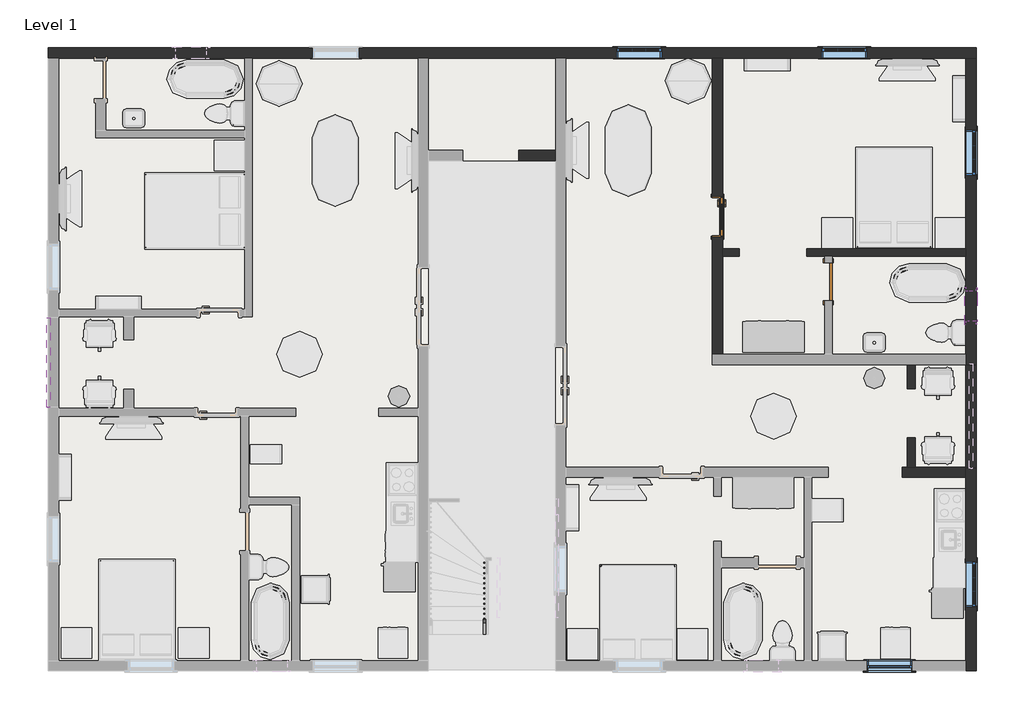
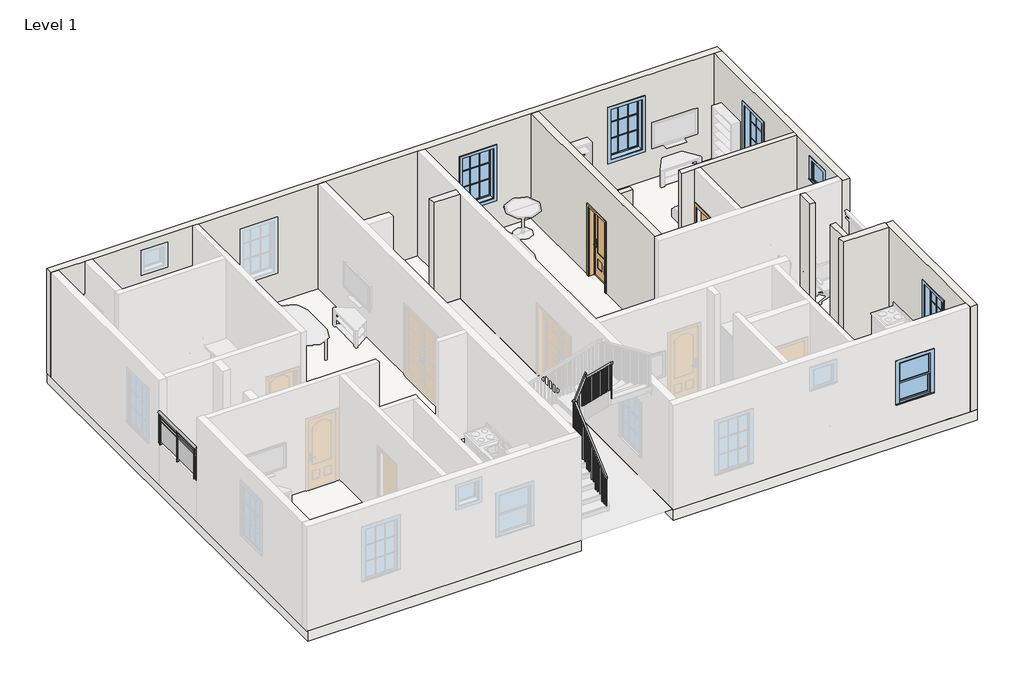
# One storey, part 2 of 4: 11 walls, 6 windows, 2 doors, 2 railings, 1 slab.
"""IFC4 building model written with IfcOpenShell, lengths in millimetres."""

from ifc_helpers import new_model, si_unit, point, frame, origin, origin_with_axes, place, context, project, spatial, polyline, ellipse_curve, trimmed, outline, extrude, faceted_brep, transform, mapped, element, save
from ifc_brep_helpers import plane_surface, extruded_surface, advanced_brep
from components import door_41326d50, door_255cab33, window_58e1470a, window_31198920, window_e41d21a6

model = new_model("IFC4")

# Units and contexts
model_context = context("Model", 3, world=origin())
ifc_project = project(units=[si_unit("LENGTHUNIT", "METRE", prefix="MILLI")], contexts=[model_context])

# Site, building, storey
site = spatial("IfcSite", under=ifc_project)
building = spatial("IfcBuilding", under=site)
storey = spatial("IfcBuildingStorey", under=building, Name="Level 1", Elevation=0.0)

# Doors
placement = place(None, origin())
door_shape = door_41326d50(model_context)
element("IfcDoor", 1, ObjectType="30\" x 80\"", at=placement, inside=storey, context=model_context, shape_type="MappedRepresentation", body=[
    mapped(door_shape, transform((-3299.0058972, 9528.0923354, 0.0), x_axis=(0.0, 1.0, 0.0), y_axis=(-1.0, 0.0, 0.0), z_axis=(0.0, 0.0, 1.0))),
])
door_2_shape = door_255cab33(model_context)
element("IfcDoor", 2, ObjectType="Single-Flush : 30\" x 80\"", at=placement, inside=storey, context=model_context, shape_type="MappedRepresentation", body=[
    mapped(door_2_shape, transform((-1092.3808972, 8232.6923354, 0.0), x_axis=(0.0, 1.0, 0.0), y_axis=(-1.0, 0.0, 0.0), z_axis=(0.0, 0.0, 1.0))),
])

# Railings
element("IfcRailing", 3, ObjectType="Glass Panel - Bottom Fill", at=placement, inside=storey, context=model_context, shape_type="SolidModel", body=[
    advanced_brep(
    [(-16599.0808972, 7508.7923354, 2133.6), (-16675.2808972, 7508.7923354, 2133.6), (-16599.0808972, 5730.7923354, 2133.6), (-16675.2808972, 5730.7923354, 2133.6)],
    [
        (0, 1, ellipse_curve(frame((-16637.1808972, 7508.7923354, 2133.6), z_axis=(0.0, 1.0, 0.0), x_axis=(-1.0, 0.0, 0.0)), 38.1, 28.575)),
        (1, 0, ellipse_curve(frame((-16637.1808972, 7508.7923354, 2133.6), z_axis=(0.0, 1.0, 0.0), x_axis=(-1.0, 0.0, 0.0)), 38.1, 28.575)),
        (2, 3, ellipse_curve(frame((-16637.1808972, 5730.7923354, 2133.6), z_axis=(0.0, -1.0, 0.0), x_axis=(-1.0, 0.0, 0.0)), 38.1, 28.575)),
        (3, 2, ellipse_curve(frame((-16637.1808972, 5730.7923354, 2133.6), z_axis=(0.0, -1.0, 0.0), x_axis=(-1.0, 0.0, 0.0)), 38.1, 28.575)),
        (0, 2),
        (3, 1),
    ],
    [
        plane_surface(frame((-16637.1808972, 7508.7923354, 2133.6), z_axis=(0.0, 1.0, 0.0), x_axis=(0.0, 0.0, -1.0))),
        plane_surface(frame((-16637.1808972, 5730.7923354, 2133.6), z_axis=(0.0, -1.0, 0.0), x_axis=(0.0, 0.0, -1.0))),
        extruded_surface(trimmed(ellipse_curve(frame((-16637.1808972, 5730.7923354, 2133.6), z_axis=(0.0, 1.0, 0.0), x_axis=(-1.0, 0.0, 0.0)), 38.1, 28.575), [point((-16599.0808972, 5730.7923354, 2133.6))], [point((-16675.2808972, 5730.7923354, 2133.6))], True, "CARTESIAN"), (0.0, 1778.0, 0.0), 1778.0),
        extruded_surface(trimmed(ellipse_curve(frame((-16637.1808972, 5730.7923354, 2133.6), z_axis=(0.0, 1.0, 0.0), x_axis=(-1.0, 0.0, 0.0)), 38.1, 28.575), [point((-16675.2808972, 5730.7923354, 2133.6))], [point((-16599.0808972, 5730.7923354, 2133.6))], True, "CARTESIAN"), (0.0, 1778.0, 0.0), 1778.0),
    ],
    [
        (0, [[1, 2]]),
        (1, [[3, 4]]),
        (2, [[-1, 5, -4, 6]]),
        (3, [[-2, -6, -3, -5]]),
    ],
),
    extrude(outline(polyline([(-16649.8808972, 7508.7923354), (-16624.4808972, 7508.7923354), (-16624.4808972, 5730.7923354), (-16649.8808972, 5730.7923354), (-16649.8808972, 7508.7923354)])), frame((0.0, 0.0, 2019.3), z_axis=(0.0, 0.0, 1.0), x_axis=(1.0, 0.0, 0.0)), (0.0, 0.0, 1.0), 25.4),
    extrude(outline(polyline([(-16649.8808972, 7508.7923354), (-16624.4808972, 7508.7923354), (-16624.4808972, 5730.7923354), (-16649.8808972, 5730.7923354), (-16649.8808972, 7508.7923354)])), frame((0.0, 0.0, 1917.7), z_axis=(0.0, 0.0, 1.0), x_axis=(1.0, 0.0, 0.0)), (0.0, 0.0, 1.0), 25.4),
    extrude(outline(polyline([(-16662.5808972, 5813.3423354), (-16611.7808972, 5813.3423354), (-16611.7808972, 5800.6423354), (-16662.5808972, 5800.6423354), (-16662.5808972, 5813.3423354)])), frame((0.0, 0.0, 1219.2), z_axis=(0.0, 0.0, 1.0), x_axis=(1.0, 0.0, 0.0)), (0.0, 0.0, 1.0), 885.6788223),
    extrude(outline(polyline([(-16630.6457402, 6619.7923354), (-16630.6457402, 5806.9923354), (-16636.9957402, 5806.9923354), (-16636.9957402, 6619.7923354), (-16630.6457402, 6619.7923354)])), frame((0.0, 0.0, 1320.8), z_axis=(0.0, 0.0, 1.0), x_axis=(1.0, 0.0, 0.0)), (0.0, 0.0, 1.0), 596.9),
    extrude(outline(polyline([(-16662.5808972, 6626.1423354), (-16611.7808972, 6626.1423354), (-16611.7808972, 6613.4423354), (-16662.5808972, 6613.4423354), (-16662.5808972, 6626.1423354)])), frame((0.0, 0.0, 1219.2), z_axis=(0.0, 0.0, 1.0), x_axis=(1.0, 0.0, 0.0)), (0.0, 0.0, 1.0), 885.6788223),
    extrude(outline(polyline([(-16630.6457402, 7432.5923354), (-16630.6457402, 6619.7923354), (-16636.9957402, 6619.7923354), (-16636.9957402, 7432.5923354), (-16630.6457402, 7432.5923354)])), frame((0.0, 0.0, 1320.8), z_axis=(0.0, 0.0, 1.0), x_axis=(1.0, 0.0, 0.0)), (0.0, 0.0, 1.0), 596.9),
    extrude(outline(polyline([(-16662.5808972, 7438.9423354), (-16611.7808972, 7438.9423354), (-16611.7808972, 7426.2423354), (-16662.5808972, 7426.2423354), (-16662.5808972, 7438.9423354)])), frame((0.0, 0.0, 1219.2), z_axis=(0.0, 0.0, 1.0), x_axis=(1.0, 0.0, 0.0)), (0.0, 0.0, 1.0), 885.6788223),
    extrude(outline(polyline([(-16646.7058972, 5743.4923354), (-16627.6558972, 5743.4923354), (-16627.6558972, 5724.4423354), (-16646.7058972, 5724.4423354), (-16646.7058972, 5743.4923354)])), frame((0.0, 0.0, 1219.2), z_axis=(0.0, 0.0, 1.0), x_axis=(1.0, 0.0, 0.0)), (0.0, 0.0, 1.0), 885.6788223),
    extrude(outline(polyline([(-16646.7058972, 7515.1423354), (-16627.6558972, 7515.1423354), (-16627.6558972, 7496.0923354), (-16646.7058972, 7496.0923354), (-16646.7058972, 7515.1423354)])), frame((0.0, 0.0, 1219.2), z_axis=(0.0, 0.0, 1.0), x_axis=(1.0, 0.0, 0.0)), (0.0, 0.0, 1.0), 885.6788223),
])
element("IfcRailing", 4, ObjectType="Handrail - Rectangular", at=placement, inside=storey, context=model_context, shape_type="SolidModel", body=[
    faceted_brep([(-7975.7808972, 1205.8606436, 1009.7665352), (-7975.7808972, 1205.8606436, 942.4055822), (-7924.9808972, 1205.8606436, 942.4055822), (-7924.9808972, 1205.8606436, 1009.7665352), (-7975.7808972, 2691.0372788, 2303.0509683), (-7975.7808972, 2710.0554775, 2252.2509683), (-7924.9808972, 2710.0554775, 2252.2509683), (-7924.9808972, 2691.0372788, 2303.0509683), (-7975.7808972, 2784.3923354, 2303.0509683), (-7924.9808972, 2784.3923354, 2303.0509683), (-7924.9808972, 2784.3923354, 2252.2509683), (-7975.7808972, 2784.3923354, 2252.2509683)], [[[0, 1, 2, 3]], [[1, 0, 4, 5]], [[2, 1, 5, 6]], [[3, 2, 6, 7]], [[0, 3, 7, 4]], [[8, 9, 10, 11]], [[5, 4, 8, 11]], [[6, 5, 11, 10]], [[7, 6, 10, 9]], [[4, 7, 9, 8]]]),
    faceted_brep([(-7924.9808972, 2784.3923354, 2302.4107175), (-7924.9808972, 2784.3923354, 2174.7946033), (-7924.9808972, 2733.5923354, 2174.7946033), (-7924.9808972, 2733.5923354, 2302.4107175), (-7620.1808972, 2784.3923354, 3004.8268147), (-7620.1808972, 2733.5923354, 3004.8268147), (-7620.1808972, 2733.5923354, 2877.2107005), (-7620.1808972, 2784.3923354, 2877.2107005)], [[[0, 1, 2, 3]], [[4, 5, 6, 7]], [[1, 0, 4, 7]], [[2, 1, 7, 6]], [[3, 2, 6, 5]], [[0, 3, 5, 4]]]),
    faceted_brep([(-7594.7808972, 2758.9923354, 2941.2311962), (-7594.7808972, 2758.9923354, 2890.4311962), (-7645.5808972, 2758.9923354, 2890.4311962), (-7645.5808972, 2758.9923354, 2941.2311962), (-7594.7808972, 2692.9950238, 2941.2311962), (-7594.7808972, 2672.5023112, 2890.4311962), (-7645.5808972, 2672.5023112, 2890.4311962), (-7645.5808972, 2692.9950238, 2941.2311962), (-7594.7808972, 1529.5899254, 4062.299085), (-7645.5808972, 1529.5899254, 4062.299085), (-7645.5808972, 1529.5899254, 3991.752118), (-7594.7808972, 1529.5899254, 3991.752118)], [[[0, 1, 2, 3]], [[1, 0, 4, 5]], [[2, 1, 5, 6]], [[3, 2, 6, 7]], [[0, 3, 7, 4]], [[8, 9, 10, 11]], [[5, 4, 8, 11]], [[6, 5, 11, 10]], [[7, 6, 10, 9]], [[4, 7, 9, 8]]]),
    extrude(outline(polyline([(1565.8700238, 3956.7922804), (1584.9200238, 3938.4355246), (1584.9200238, 2878.6666667), (1565.8700238, 2878.6666667), (1565.8700238, 3956.7922804)])), frame((-7629.7058972, 0.0, 0.0), z_axis=(1.0, 0.0, 0.0), x_axis=(0.0, 1.0, 0.0)), (0.0, 0.0, 1.0), 19.05),
    extrude(outline(polyline([(1667.4700238, 3858.8895829), (1686.5200238, 3840.5328271), (1686.5200238, 2878.6666667), (1667.4700238, 2878.6666667), (1667.4700238, 3858.8895829)])), frame((-7629.7058972, 0.0, 0.0), z_axis=(1.0, 0.0, 0.0), x_axis=(0.0, 1.0, 0.0)), (0.0, 0.0, 1.0), 19.05),
    extrude(outline(polyline([(1769.0700238, 3760.9868853), (1788.1200238, 3742.6301295), (1788.1200238, 2878.6666667), (1769.0700238, 2878.6666667), (1769.0700238, 3760.9868853)])), frame((-7629.7058972, 0.0, 0.0), z_axis=(1.0, 0.0, 0.0), x_axis=(0.0, 1.0, 0.0)), (0.0, 0.0, 1.0), 19.05),
    extrude(outline(polyline([(1870.6700238, 3663.0841877), (1889.7200238, 3644.7274319), (1889.7200238, 2709.3333333), (1870.6700238, 2709.3333333), (1870.6700238, 3663.0841877)])), frame((-7629.7058972, 0.0, 0.0), z_axis=(1.0, 0.0, 0.0), x_axis=(0.0, 1.0, 0.0)), (0.0, 0.0, 1.0), 19.05),
    extrude(outline(polyline([(1972.2700238, 3565.1814902), (1991.3200238, 3546.8247344), (1991.3200238, 2709.3333333), (1972.2700238, 2709.3333333), (1972.2700238, 3565.1814902)])), frame((-7629.7058972, 0.0, 0.0), z_axis=(1.0, 0.0, 0.0), x_axis=(0.0, 1.0, 0.0)), (0.0, 0.0, 1.0), 19.05),
    extrude(outline(polyline([(2073.8700238, 3467.2787926), (2092.9200238, 3448.9220368), (2092.9200238, 2709.3333333), (2073.8700238, 2709.3333333), (2073.8700238, 3467.2787926)])), frame((-7629.7058972, 0.0, 0.0), z_axis=(1.0, 0.0, 0.0), x_axis=(0.0, 1.0, 0.0)), (0.0, 0.0, 1.0), 19.05),
    extrude(outline(polyline([(2175.4700238, 3369.376095), (2194.5200238, 3351.0193392), (2194.5200238, 2540.0), (2175.4700238, 2540.0), (2175.4700238, 3369.376095)])), frame((-7629.7058972, 0.0, 0.0), z_axis=(1.0, 0.0, 0.0), x_axis=(0.0, 1.0, 0.0)), (0.0, 0.0, 1.0), 19.05),
    extrude(outline(polyline([(2277.0700238, 3271.4733974), (2296.1200238, 3253.1166416), (2296.1200238, 2370.6666667), (2277.0700238, 2370.6666667), (2277.0700238, 3271.4733974)])), frame((-7629.7058972, 0.0, 0.0), z_axis=(1.0, 0.0, 0.0), x_axis=(0.0, 1.0, 0.0)), (0.0, 0.0, 1.0), 19.05),
    extrude(outline(polyline([(2378.6700238, 3173.5706999), (2397.7200238, 3155.2139441), (2397.7200238, 2370.6666667), (2378.6700238, 2370.6666667), (2378.6700238, 3173.5706999)])), frame((-7629.7058972, 0.0, 0.0), z_axis=(1.0, 0.0, 0.0), x_axis=(0.0, 1.0, 0.0)), (0.0, 0.0, 1.0), 19.05),
    extrude(outline(polyline([(2480.2700238, 3075.6680023), (2499.3200238, 3057.3112465), (2499.3200238, 2201.3333333), (2480.2700238, 2201.3333333), (2480.2700238, 3075.6680023)])), frame((-7629.7058972, 0.0, 0.0), z_axis=(1.0, 0.0, 0.0), x_axis=(0.0, 1.0, 0.0)), (0.0, 0.0, 1.0), 19.05),
    extrude(outline(polyline([(2581.8700238, 2977.7653047), (2600.9200238, 2959.4085489), (2600.9200238, 2032.0), (2581.8700238, 2032.0), (2581.8700238, 2977.7653047)])), frame((-7629.7058972, 0.0, 0.0), z_axis=(1.0, 0.0, 0.0), x_axis=(0.0, 1.0, 0.0)), (0.0, 0.0, 1.0), 19.05),
    extrude(outline(polyline([(2665.6627553, -7711.9780726), (2621.7617492, -7731.0280726), (1693.3333333, -7731.0280726), (1693.3333333, -7711.9780726), (2665.6627553, -7711.9780726)])), frame((0.0, 2749.4673354, 0.0), z_axis=(0.0, 1.0, 0.0), x_axis=(0.0, 0.0, 1.0)), (0.0, 0.0, 1.0), 19.05),
    extrude(outline(polyline([(2431.5240562, -7813.5780726), (2387.6230501, -7832.6280726), (1524.0, -7832.6280726), (1524.0, -7813.5780726), (2431.5240562, -7813.5780726)])), frame((0.0, 2749.4673354, 0.0), z_axis=(0.0, 1.0, 0.0), x_axis=(0.0, 0.0, 1.0)), (0.0, 0.0, 1.0), 19.05),
    extrude(outline(polyline([(2618.7356436, 2172.7301107), (2637.7856436, 2189.318756), (2637.7856436, 1185.3333333), (2618.7356436, 1185.3333333), (2618.7356436, 2172.7301107)])), frame((-7959.9058972, 0.0, 0.0), z_axis=(1.0, 0.0, 0.0), x_axis=(0.0, 1.0, 0.0)), (0.0, 0.0, 1.0), 19.05),
    extrude(outline(polyline([(2517.1356436, 2084.2573356), (2536.1856436, 2100.8459809), (2536.1856436, 1185.3333333), (2517.1356436, 1185.3333333), (2517.1356436, 2084.2573356)])), frame((-7959.9058972, 0.0, 0.0), z_axis=(1.0, 0.0, 0.0), x_axis=(0.0, 1.0, 0.0)), (0.0, 0.0, 1.0), 19.05),
    extrude(outline(polyline([(2415.5356436, 1995.7845605), (2434.5856436, 2012.3732059), (2434.5856436, 1016.0), (2415.5356436, 1016.0), (2415.5356436, 1995.7845605)])), frame((-7959.9058972, 0.0, 0.0), z_axis=(1.0, 0.0, 0.0), x_axis=(0.0, 1.0, 0.0)), (0.0, 0.0, 1.0), 19.05),
    extrude(outline(polyline([(2313.9356436, 1907.3117855), (2332.9856436, 1923.9004308), (2332.9856436, 846.6666667), (2313.9356436, 846.6666667), (2313.9356436, 1907.3117855)])), frame((-7959.9058972, 0.0, 0.0), z_axis=(1.0, 0.0, 0.0), x_axis=(0.0, 1.0, 0.0)), (0.0, 0.0, 1.0), 19.05),
    extrude(outline(polyline([(2212.3356436, 1818.8390104), (2231.3856436, 1835.4276557), (2231.3856436, 846.6666667), (2212.3356436, 846.6666667), (2212.3356436, 1818.8390104)])), frame((-7959.9058972, 0.0, 0.0), z_axis=(1.0, 0.0, 0.0), x_axis=(0.0, 1.0, 0.0)), (0.0, 0.0, 1.0), 19.05),
    extrude(outline(polyline([(2110.7356436, 1730.3662353), (2129.7856436, 1746.9548806), (2129.7856436, 677.3333333), (2110.7356436, 677.3333333), (2110.7356436, 1730.3662353)])), frame((-7959.9058972, 0.0, 0.0), z_axis=(1.0, 0.0, 0.0), x_axis=(0.0, 1.0, 0.0)), (0.0, 0.0, 1.0), 19.05),
    extrude(outline(polyline([(2009.1356436, 1641.8934602), (2028.1856436, 1658.4821055), (2028.1856436, 677.3333333), (2009.1356436, 677.3333333), (2009.1356436, 1641.8934602)])), frame((-7959.9058972, 0.0, 0.0), z_axis=(1.0, 0.0, 0.0), x_axis=(0.0, 1.0, 0.0)), (0.0, 0.0, 1.0), 19.05),
    extrude(outline(polyline([(1907.5356436, 1553.4206851), (1926.5856436, 1570.0093305), (1926.5856436, 508.0), (1907.5356436, 508.0), (1907.5356436, 1553.4206851)])), frame((-7959.9058972, 0.0, 0.0), z_axis=(1.0, 0.0, 0.0), x_axis=(0.0, 1.0, 0.0)), (0.0, 0.0, 1.0), 19.05),
    extrude(outline(polyline([(1805.9356436, 1464.9479101), (1824.9856436, 1481.5365554), (1824.9856436, 508.0), (1805.9356436, 508.0), (1805.9356436, 1464.9479101)])), frame((-7959.9058972, 0.0, 0.0), z_axis=(1.0, 0.0, 0.0), x_axis=(0.0, 1.0, 0.0)), (0.0, 0.0, 1.0), 19.05),
    extrude(outline(polyline([(1704.3356436, 1376.475135), (1723.3856436, 1393.0637803), (1723.3856436, 338.6666667), (1704.3356436, 338.6666667), (1704.3356436, 1376.475135)])), frame((-7959.9058972, 0.0, 0.0), z_axis=(1.0, 0.0, 0.0), x_axis=(0.0, 1.0, 0.0)), (0.0, 0.0, 1.0), 19.05),
    extrude(outline(polyline([(1602.7356436, 1288.0023599), (1621.7856436, 1304.5910052), (1621.7856436, 338.6666667), (1602.7356436, 338.6666667), (1602.7356436, 1288.0023599)])), frame((-7959.9058972, 0.0, 0.0), z_axis=(1.0, 0.0, 0.0), x_axis=(0.0, 1.0, 0.0)), (0.0, 0.0, 1.0), 19.05),
    extrude(outline(polyline([(1501.1356436, 1199.5295848), (1520.1856436, 1216.1182301), (1520.1856436, 338.6666667), (1501.1356436, 338.6666667), (1501.1356436, 1199.5295848)])), frame((-7959.9058972, 0.0, 0.0), z_axis=(1.0, 0.0, 0.0), x_axis=(0.0, 1.0, 0.0)), (0.0, 0.0, 1.0), 19.05),
    extrude(outline(polyline([(1399.5356436, 1111.0568097), (1418.5856436, 1127.6454551), (1418.5856436, 169.3333333), (1399.5356436, 169.3333333), (1399.5356436, 1111.0568097)])), frame((-7959.9058972, 0.0, 0.0), z_axis=(1.0, 0.0, 0.0), x_axis=(0.0, 1.0, 0.0)), (0.0, 0.0, 1.0), 19.05),
    extrude(outline(polyline([(1297.9356436, 1022.5840347), (1316.9856436, 1039.17268), (1316.9856436, 169.3333333), (1297.9356436, 169.3333333), (1297.9356436, 1022.5840347)])), frame((-7959.9058972, 0.0, 0.0), z_axis=(1.0, 0.0, 0.0), x_axis=(0.0, 1.0, 0.0)), (0.0, 0.0, 1.0), 19.05),
    extrude(outline(polyline([(-7629.7058972, 2702.5200238), (-7610.6558972, 2702.5200238), (-7610.6558972, 2683.4700238), (-7629.7058972, 2683.4700238), (-7629.7058972, 2702.5200238)])), frame((0.0, 0.0, 2032.0), z_axis=(0.0, 0.0, 1.0), x_axis=(1.0, 0.0, 0.0)), (0.0, 0.0, 1.0), 858.4311962),
    extrude(outline(polyline([(2899.1612036, -7610.6558972), (2855.2601975, -7629.7058972), (1862.6666667, -7629.7058972), (1862.6666667, -7610.6558972), (2899.1612036, -7610.6558972)])), frame((0.0, 2749.4673354, 0.0), z_axis=(0.0, 1.0, 0.0), x_axis=(0.0, 0.0, 1.0)), (0.0, 0.0, 1.0), 19.05),
    extrude(outline(polyline([(2835.5655851, -7638.2519967), (2791.664579, -7657.3019967), (1862.6666667, -7657.3019967), (1862.6666667, -7638.2519967), (2835.5655851, -7638.2519967)])), frame((0.0, 2749.4673354, 0.0), z_axis=(0.0, 1.0, 0.0), x_axis=(0.0, 0.0, 1.0)), (0.0, 0.0, 1.0), 19.05),
    extrude(outline(polyline([(2197.3853571, -7915.1780726), (2153.484351, -7934.2280726), (1354.6666667, -7934.2280726), (1354.6666667, -7915.1780726), (2197.3853571, -7915.1780726)])), frame((0.0, 2749.4673354, 0.0), z_axis=(0.0, 1.0, 0.0), x_axis=(0.0, 0.0, 1.0)), (0.0, 0.0, 1.0), 19.05),
    extrude(outline(polyline([(-7940.8558972, 2749.4673354), (-7959.9058972, 2749.4673354), (-7959.9058972, 2768.5173354), (-7940.8558972, 2768.5173354), (-7940.8558972, 2749.4673354)])), frame((0.0, 0.0, 1354.6666667), z_axis=(0.0, 0.0, 1.0), x_axis=(1.0, 0.0, 0.0)), (0.0, 0.0, 1.0), 897.5843016),
    extrude(outline(polyline([(2681.5122788, 2227.3956927), (2700.5622788, 2243.984338), (2700.5622788, 1354.6666667), (2681.5122788, 1354.6666667), (2681.5122788, 2227.3956927)])), frame((-7959.9058972, 0.0, 0.0), z_axis=(1.0, 0.0, 0.0), x_axis=(0.0, 1.0, 0.0)), (0.0, 0.0, 1.0), 19.05),
    extrude(outline(polyline([(1529.5899254, 3991.752118), (1548.6399254, 3973.3953622), (1548.6399254, 2878.6666667), (1529.5899254, 2878.6666667), (1529.5899254, 3991.752118)])), frame((-7629.7058972, 0.0, 0.0), z_axis=(1.0, 0.0, 0.0), x_axis=(0.0, 1.0, 0.0)), (0.0, 0.0, 1.0), 19.05),
    extrude(outline(polyline([(1205.8606436, 942.4055822), (1224.9106436, 958.9942276), (1224.9106436, 169.3333333), (1205.8606436, 169.3333333), (1205.8606436, 942.4055822)])), frame((-7959.9058972, 0.0, 0.0), z_axis=(1.0, 0.0, 0.0), x_axis=(0.0, 1.0, 0.0)), (0.0, 0.0, 1.0), 19.05),
])

# Slab
element("IfcSlab", 5, ObjectType="Generic - 12\"", at=placement, inside=storey, context=model_context, shape_type="SweptSolid", body=[
    extrude(outline(polyline([(-16611.7808972, 472.9923354), (-16611.7808972, 12893.5923354), (1854.0191028, 12893.5923354), (1854.0191028, 472.9923354), (-6527.9808972, 472.9923354), (-6527.9808972, 10645.6923354), (-9067.9808972, 10645.6923354), (-9067.9808972, 472.9923354), (-16611.7808972, 472.9923354)])), frame((0.0, 0.0, -304.8), z_axis=(0.0, 0.0, 1.0), x_axis=(1.0, 0.0, 0.0)), (0.0, 0.0, 1.0), 304.8),
])

# Walls
element("IfcWall", 6, ObjectType="Generic - 8\"", at=placement, inside=storey, context=model_context, shape_type="Brep", body=[
    faceted_brep([(-16637.1808972, 12690.3923354, 0.0), (-16433.9808972, 12690.3923354, 0.0), (-15697.3808972, 12690.3923354, 0.0), (-15494.1808972, 12690.3923354, 0.0), (-12725.5808972, 12690.3923354, 0.0), (-12573.1808972, 12690.3923354, 0.0), (-9271.1808972, 12690.3923354, 0.0), (-9067.9808972, 12690.3923354, 0.0), (-6527.9808972, 12690.3923354, 0.0), (-6324.7808972, 12690.3923354, 0.0), (-3403.7808972, 12690.3923354, 0.0), (-3200.5808972, 12690.3923354, 0.0), (1650.8191028, 12690.3923354, 0.0), (1854.0191028, 12690.3923354, 0.0), (1854.0191028, 12690.3923354, 3048.0), (1650.8191028, 12690.3923354, 3048.0), (-3200.5808972, 12690.3923354, 3048.0), (-3403.7808972, 12690.3923354, 3048.0), (-6324.7808972, 12690.3923354, 3048.0), (-6527.9808972, 12690.3923354, 3048.0), (-9067.9808972, 12690.3923354, 3048.0), (-9271.1808972, 12690.3923354, 3048.0), (-12573.1808972, 12690.3923354, 3048.0), (-12725.5808972, 12690.3923354, 3048.0), (-15494.1808972, 12690.3923354, 3048.0), (-15697.3808972, 12690.3923354, 3048.0), (-16433.9808972, 12690.3923354, 3048.0), (-16637.1808972, 12690.3923354, 3048.0), (-10452.2808972, 12690.3923354, 2438.4), (-10452.2808972, 12690.3923354, 914.4), (-11366.6808972, 12690.3923354, 914.4), (-11366.6808972, 12690.3923354, 2438.4), (-4407.0808972, 12690.3923354, 2438.4), (-4407.0808972, 12690.3923354, 914.4), (-5321.4808972, 12690.3923354, 914.4), (-5321.4808972, 12690.3923354, 2438.4), (-317.6808972, 12690.3923354, 2438.4), (-317.6808972, 12690.3923354, 914.4), (-1232.0808972, 12690.3923354, 914.4), (-1232.0808972, 12690.3923354, 2438.4), (-13487.5808972, 12690.3923354, 2768.6), (-13487.5808972, 12690.3923354, 2159.0), (-14097.1808972, 12690.3923354, 2159.0), (-14097.1808972, 12690.3923354, 2768.6), (-16637.1808972, 12893.5923354, 0.0), (-16637.1808972, 12893.5923354, 3048.0), (1854.0191028, 12893.5923354, 3048.0), (1854.0191028, 12893.5923354, 0.0), (-10452.2808972, 12893.5923354, 2438.4), (-11366.6808972, 12893.5923354, 2438.4), (-11366.6808972, 12893.5923354, 914.4), (-10452.2808972, 12893.5923354, 914.4), (-4407.0808972, 12893.5923354, 2438.4), (-5321.4808972, 12893.5923354, 2438.4), (-5321.4808972, 12893.5923354, 914.4), (-4407.0808972, 12893.5923354, 914.4), (-317.6808972, 12893.5923354, 2438.4), (-1232.0808972, 12893.5923354, 2438.4), (-1232.0808972, 12893.5923354, 914.4), (-317.6808972, 12893.5923354, 914.4), (-13487.5808972, 12893.5923354, 2768.6), (-14097.1808972, 12893.5923354, 2768.6), (-14097.1808972, 12893.5923354, 2159.0), (-13487.5808972, 12893.5923354, 2159.0)], [[[0, 1, 2, 3, 4, 5, 6, 7, 8, 9, 10, 11, 12, 13, 14, 15, 16, 17, 18, 19, 20, 21, 22, 23, 24, 25, 26, 27], [28, 29, 30, 31], [32, 33, 34, 35], [36, 37, 38, 39], [40, 41, 42, 43]], [[44, 45, 46, 47], [48, 49, 50, 51], [52, 53, 54, 55], [56, 57, 58, 59], [60, 61, 62, 63]], [[13, 12, 11, 10, 9, 8, 7, 6, 5, 4, 3, 2, 1, 0, 44, 47]], [[27, 26, 25, 24, 23, 22, 21, 20, 19, 18, 17, 16, 15, 14, 46, 45]], [[14, 13, 47, 46]], [[0, 27, 45, 44]], [[29, 28, 48, 51]], [[30, 29, 51, 50]], [[31, 30, 50, 49]], [[28, 31, 49, 48]], [[33, 32, 52, 55]], [[34, 33, 55, 54]], [[35, 34, 54, 53]], [[32, 35, 53, 52]], [[37, 36, 56, 59]], [[38, 37, 59, 58]], [[39, 38, 58, 57]], [[36, 39, 57, 56]], [[41, 40, 60, 63]], [[42, 41, 63, 62]], [[43, 42, 62, 61]], [[40, 43, 61, 60]]]),
])
element("IfcWall", 7, ObjectType="Generic - 8\"", at=placement, inside=storey, context=model_context, shape_type="Brep", body=[
    faceted_brep([(1650.8191028, 12690.3923354, 0.0), (1650.8191028, 8893.0923354, 0.0), (1650.8191028, 8740.6923354, 0.0), (1650.8191028, 6784.8923354, 0.0), (1650.8191028, 6581.6923354, 0.0), (1650.8191028, 6568.9923354, 0.0), (1650.8191028, 6568.9923354, 1219.2), (1650.8191028, 6568.9923354, 3048.0), (1650.8191028, 6581.6923354, 3048.0), (1650.8191028, 6784.8923354, 3048.0), (1650.8191028, 8740.6923354, 3048.0), (1650.8191028, 8893.0923354, 3048.0), (1650.8191028, 12690.3923354, 3048.0), (1650.8191028, 10347.2423354, 2438.4), (1650.8191028, 10347.2423354, 914.4), (1650.8191028, 11261.6423354, 914.4), (1650.8191028, 11261.6423354, 2438.4), (1650.8191028, 8054.8923354, 2768.6), (1650.8191028, 7445.2923354, 2768.6), (1650.8191028, 7445.2923354, 2159.0), (1650.8191028, 8054.8923354, 2159.0), (1854.0191028, 12690.3923354, 0.0), (1854.0191028, 12690.3923354, 3048.0), (1854.0191028, 6568.9923354, 3048.0), (1854.0191028, 6568.9923354, 1219.2), (1854.0191028, 6568.9923354, 0.0), (1854.0191028, 10347.2423354, 2438.4), (1854.0191028, 11261.6423354, 2438.4), (1854.0191028, 11261.6423354, 914.4), (1854.0191028, 10347.2423354, 914.4), (1854.0191028, 8054.8923354, 2768.6), (1854.0191028, 8054.8923354, 2159.0), (1854.0191028, 7445.2923354, 2159.0), (1854.0191028, 7445.2923354, 2768.6)], [[[0, 1, 2, 3, 4, 5, 6, 7, 8, 9, 10, 11, 12], [13, 14, 15, 16], [17, 18, 19, 20]], [[21, 22, 23, 24, 25], [26, 27, 28, 29], [30, 31, 32, 33]], [[5, 4, 3, 2, 1, 0, 21, 25]], [[7, 6, 5, 25, 24, 23]], [[12, 11, 10, 9, 8, 7, 23, 22]], [[0, 12, 22, 21]], [[14, 13, 26, 29]], [[15, 14, 29, 28]], [[16, 15, 28, 27]], [[13, 16, 27, 26]], [[31, 30, 17, 20]], [[32, 31, 20, 19]], [[33, 32, 19, 18]], [[30, 33, 18, 17]]]),
])
element("IfcWall", 8, ObjectType="Generic - 8\"", at=placement, inside=storey, context=model_context, shape_type="Brep", body=[
    faceted_brep([(-3200.5808972, 12690.3923354, 3048.0), (-3200.5808972, 8893.0923354, 3048.0), (-3200.5808972, 8740.6923354, 3048.0), (-3200.5808972, 6784.8923354, 3048.0), (-3200.5808972, 6784.8923354, 0.0), (-3200.5808972, 8740.6923354, 0.0), (-3200.5808972, 8893.0923354, 0.0), (-3200.5808972, 9121.6923354, 0.0), (-3200.5808972, 9121.6923354, 2057.4), (-3200.5808972, 9934.4923354, 2057.4), (-3200.5808972, 9934.4923354, 0.0), (-3200.5808972, 12690.3923354, 0.0), (-3403.7808972, 6784.8923354, 3048.0), (-3403.7808972, 12690.3923354, 3048.0), (-3403.7808972, 12690.3923354, 0.0), (-3403.7808972, 9934.4923354, 0.0), (-3403.7808972, 9934.4923354, 2057.4), (-3403.7808972, 9121.6923354, 2057.4), (-3403.7808972, 9121.6923354, 0.0), (-3403.7808972, 6784.8923354, 0.0)], [[[0, 1, 2, 3, 4, 5, 6, 7, 8, 9, 10, 11]], [[12, 13, 14, 15, 16, 17, 18, 19]], [[4, 19, 18, 7, 6, 5]], [[14, 11, 10, 15]], [[3, 2, 1, 0, 13, 12]], [[4, 3, 12, 19]], [[0, 11, 14, 13]], [[9, 16, 15, 10]], [[16, 9, 8, 17]], [[17, 8, 7, 18]]]),
])
element("IfcWall", 9, ObjectType="Generic - 8\"", at=placement, inside=storey, context=model_context, shape_type="Brep", body=[
    faceted_brep([(380.8191028, 4333.7923354, 0.0), (1650.8191028, 4333.7923354, 0.0), (1650.8191028, 4333.7923354, 3048.0), (380.8191028, 4333.7923354, 3048.0), (380.8191028, 4536.9923354, 0.0), (380.8191028, 4536.9923354, 3048.0), (482.4191028, 4536.9923354, 3048.0), (634.8191028, 4536.9923354, 3048.0), (1650.8191028, 4536.9923354, 3048.0), (1650.8191028, 4536.9923354, 0.0), (634.8191028, 4536.9923354, 0.0), (482.4191028, 4536.9923354, 0.0), (1650.8191028, 4511.5923354, 0.0), (1650.8191028, 4511.5923354, 3048.0)], [[[0, 1, 2, 3]], [[4, 5, 6, 7, 8, 9, 10, 11]], [[1, 0, 4, 11, 10, 9, 12]], [[3, 2, 13, 8, 7, 6, 5]], [[0, 3, 5, 4]], [[1, 12, 9, 8, 13, 2]]]),
])
element("IfcWall", 10, ObjectType="Generic - 8\"", at=placement, inside=storey, context=model_context, shape_type="SweptSolid", body=[
    extrude(outline(polyline([(-6527.9808972, 10645.6923354), (-7264.5808972, 10645.6923354), (-7264.5808972, 10848.8923354), (-6527.9808972, 10848.8923354), (-6527.9808972, 10645.6923354)])), origin_with_axes(), (0.0, 0.0, 1.0), 3048.0),
])
element("IfcWall", 11, ObjectType="Generic - 8\"", at=placement, inside=storey, context=model_context, shape_type="Brep", body=[
    faceted_brep([(1650.8191028, 6568.9923354, 0.0), (1650.8191028, 4536.9923354, 0.0), (1650.8191028, 4511.5923354, 0.0), (1650.8191028, 4511.5923354, 1219.2), (1650.8191028, 6568.9923354, 1219.2), (1854.0191028, 6568.9923354, 0.0), (1854.0191028, 6568.9923354, 1219.2), (1854.0191028, 4511.5923354, 1219.2), (1854.0191028, 4511.5923354, 0.0)], [[[0, 1, 2, 3, 4]], [[5, 6, 7, 8]], [[2, 1, 0, 5, 8]], [[3, 2, 8, 7]], [[4, 3, 7, 6]], [[0, 4, 6, 5]]]),
])
element("IfcWall", 12, ObjectType="Generic - 8\"", at=placement, inside=storey, context=model_context, shape_type="Brep", body=[
    faceted_brep([(1650.8191028, 4511.5923354, 0.0), (1650.8191028, 4333.7923354, 0.0), (1650.8191028, 676.1923354, 0.0), (1650.8191028, 472.9923354, 0.0), (1650.8191028, 472.9923354, 3048.0), (1650.8191028, 676.1923354, 3048.0), (1650.8191028, 4333.7923354, 3048.0), (1650.8191028, 4511.5923354, 3048.0), (1650.8191028, 4511.5923354, 1219.2), (1650.8191028, 1742.9923354, 2438.4), (1650.8191028, 1742.9923354, 914.4), (1650.8191028, 2657.3923354, 914.4), (1650.8191028, 2657.3923354, 2438.4), (1854.0191028, 4511.5923354, 0.0), (1854.0191028, 4511.5923354, 1219.2), (1854.0191028, 4511.5923354, 3048.0), (1854.0191028, 472.9923354, 3048.0), (1854.0191028, 472.9923354, 0.0), (1854.0191028, 1742.9923354, 2438.4), (1854.0191028, 2657.3923354, 2438.4), (1854.0191028, 2657.3923354, 914.4), (1854.0191028, 1742.9923354, 914.4)], [[[0, 1, 2, 3, 4, 5, 6, 7, 8], [9, 10, 11, 12]], [[13, 14, 15, 16, 17], [18, 19, 20, 21]], [[3, 2, 1, 0, 13, 17]], [[7, 6, 5, 4, 16, 15]], [[0, 8, 7, 15, 14, 13]], [[4, 3, 17, 16]], [[10, 9, 18, 21]], [[11, 10, 21, 20]], [[12, 11, 20, 19]], [[9, 12, 19, 18]]]),
])
element("IfcWall", 13, ObjectType="INNER", at=placement, inside=storey, context=model_context, shape_type="SweptSolid", body=[
    extrude(outline(polyline([(-2870.3808972, 8740.6923354), (-3200.5808972, 8740.6923354), (-3200.5808972, 8893.0923354), (-2870.3808972, 8893.0923354), (-2870.3808972, 8740.6923354)])), origin_with_axes(), (0.0, 0.0, 1.0), 3048.0),
])
element("IfcWall", 14, ObjectType="INNER", at=placement, inside=storey, context=model_context, shape_type="SweptSolid", body=[
    extrude(outline(polyline([(634.8191028, 5121.1923354), (634.8191028, 4536.9923354), (482.4191028, 4536.9923354), (482.4191028, 5121.1923354), (634.8191028, 5121.1923354)])), origin_with_axes(), (0.0, 0.0, 1.0), 3048.0),
])
element("IfcWall", 15, ObjectType="INNER", at=placement, inside=storey, context=model_context, shape_type="Brep", body=[
    faceted_brep([(-1524.1808972, 8740.6923354, 0.0), (-1168.5808972, 8740.6923354, 0.0), (-1016.1808972, 8740.6923354, 0.0), (1650.8191028, 8740.6923354, 0.0), (1650.8191028, 8740.6923354, 3048.0), (-1016.1808972, 8740.6923354, 3048.0), (-1168.5808972, 8740.6923354, 3048.0), (-1524.1808972, 8740.6923354, 3048.0), (-1524.1808972, 8893.0923354, 0.0), (-1524.1808972, 8893.0923354, 3048.0), (1650.8191028, 8893.0923354, 3048.0), (1650.8191028, 8893.0923354, 0.0)], [[[0, 1, 2, 3, 4, 5, 6, 7]], [[8, 9, 10, 11]], [[3, 2, 1, 0, 8, 11]], [[7, 6, 5, 4, 10, 9]], [[0, 7, 9, 8]], [[4, 3, 11, 10]]]),
])
element("IfcWall", 16, ObjectType="INNER", at=placement, inside=storey, context=model_context, shape_type="SweptSolid", body=[
    extrude(outline(polyline([(634.8191028, 6581.6923354), (634.8191028, 6099.0923354), (482.4191028, 6099.0923354), (482.4191028, 6581.6923354), (634.8191028, 6581.6923354)])), origin_with_axes(), (0.0, 0.0, 1.0), 3048.0),
])

# Windows
window_shape = window_58e1470a(model_context)
element("IfcWindow", 17, ObjectType="Casement 3x3 with Trim : 36\" x 60\"", at=placement, inside=storey, context=model_context, shape_type="MappedRepresentation", body=[
    mapped(window_shape, transform((-4864.2808972, 12791.9923354, 304.8), x_axis=(1.0, 0.0, 0.0), y_axis=(0.0, 1.0, 0.0), z_axis=(0.0, 0.0, 1.0))),
])
element("IfcWindow", 18, ObjectType="Casement 3x3 with Trim : 36\" x 60\"", at=placement, inside=storey, context=model_context, shape_type="MappedRepresentation", body=[
    mapped(window_shape, transform((-774.8808972, 12791.9923354, 304.8), x_axis=(1.0, 0.0, 0.0), y_axis=(0.0, 1.0, 0.0), z_axis=(0.0, 0.0, 1.0))),
])
element("IfcWindow", 19, ObjectType="Casement 3x3 with Trim : 36\" x 60\"", at=placement, inside=storey, context=model_context, shape_type="MappedRepresentation", body=[
    mapped(window_shape, transform((1752.4191028, 10804.4423354, 304.8), x_axis=(0.0, -1.0, 0.0), y_axis=(1.0, 0.0, 0.0), z_axis=(0.0, 0.0, 1.0))),
])
element("IfcWindow", 20, ObjectType="Casement 3x3 with Trim : 36\" x 60\"", at=placement, inside=storey, context=model_context, shape_type="MappedRepresentation", body=[
    mapped(window_shape, transform((1752.4191028, 2200.1923354, 304.8), x_axis=(0.0, -1.0, 0.0), y_axis=(1.0, 0.0, 0.0), z_axis=(0.0, 0.0, 1.0))),
])
window_2_shape = window_31198920(model_context)
element("IfcWindow", 21, ObjectType="Double Hung with Trim : 36\" x 48\"", at=placement, inside=storey, context=model_context, shape_type="MappedRepresentation", body=[
    mapped(window_2_shape, transform((126.8191028, 574.5923354, 0.0), x_axis=(-1.0, 0.0, 0.0), y_axis=(0.0, -1.0, 0.0), z_axis=(0.0, 0.0, 1.0))),
])
window_3_shape = window_e41d21a6(model_context)
element("IfcWindow", 22, ObjectType="Transom with Trim : 24\" x 24\"", at=placement, inside=storey, context=model_context, shape_type="MappedRepresentation", body=[
    mapped(window_3_shape, transform((1752.4191028, 7788.1923354, 0.0), x_axis=(0.0, 1.0, 0.0), y_axis=(-1.0, 0.0, 0.0), z_axis=(0.0, 0.0, 1.0))),
])

save(model, "model.ifc")

# Revit data of these elements
# Type "30\" x 80\""
#   Type Mark = "8"
#   Assembly Code = "B2030100"
#   Analytic Construction = "French door, wood frame with single glass"
#   Threshold Offset [instance default] = 0' - 0 1/2"
#   Thickness = 0' - 1 3/8"
#   Thermal Resistance (R) = 1.0696 (h·ft²·°F)/BTU
#   Swing Angle [instance default] = 90.00°
#   Stiles = 0' - 4 3/4"
#   Rough Width = 2' - 8"
#   Rough Height = 6' - 9"
#   Radius = 1' - 1.00625"
#   Lock Rail = 0' - 7 1/8"
#   Height = 6' - 8"
#   Width = 2' - 6"
#   Heat Transfer Coefficient (U) = 0.9350 BTU/(h·ft²·°F)
#   Door Offset [instance default] = 0' - 0"
#   Bottom Rail = 0' - 9 1/2"
#   Threshold [instance default] = yes
#   Function = 1
#   Exterior Trim [instance default] = yes
#   Trim Material = Cherry
#   Threshold Material = Cherry
#   Panel Material = Cherry
#   Glazing = Glass
#   Frame Material = Cherry
#   Door Handle Material = Aluminum
#   Visual Light Transmittance = 0
#   Solar Heat Gain Coefficient = 0
#   Wall Closure = (empty or 0)
#   Construction Type = (empty or 0)
# Type "Single-Flush : 30\" x 80\""
#   Type Mark = "5"
#   Construction Type Id = "MDOOR"
#   Assembly Code = "C1020"
#   Analytic Construction = "Metal"
#   Thickness = 0' - 2"
#   Heat Transfer Coefficient (U) = 0.651978 BTU/(h·ft²·°F)
#   Height = 6' - 8"
#   Trim Projection Ext = 0' - 1"
#   Trim Projection Int = 0' - 1"
#   Trim Width = 0' - 3"
#   Width = 2' - 6"
#   Define Thermal Properties by = 1
#   Door Material = Door - Panel
#   Frame Material = Door - Frame
#   Visual Light Transmittance = 0
#   Solar Heat Gain Coefficient = 0
#   Function = (empty or 0)
#   Wall Closure = (empty or 0)
# Type "Glass Panel - Bottom Fill"
#   Assembly Code = "C2010400"
#   built-in parameter 1008612 = 0.0416667 (stored number, unit not read)
#   built-in parameter 1008611 = 0.0416667 (stored number, unit not read)
#   built-in parameter 1008609 = 0.333333 (stored number, unit not read)
#   built-in parameter 1008604 = 0.166667 (stored number, unit not read)
#   built-in parameter 1008603 = 0.166667 (stored number, unit not read)
#   Railing Height = 3' - 0"
#   built-in parameter 1008630 = 2
#   built-in parameter 1008610 = 2
#   built-in parameter 1008618 = Baluster - Square : 3/4"
# Type "Handrail - Rectangular"
#   Assembly Code = "C2010400"
#   built-in parameter 1008612 = 0.0416667 (stored number, unit not read)
#   built-in parameter 1008611 = 0.0416667 (stored number, unit not read)
#   built-in parameter 1008609 = 0.333333 (stored number, unit not read)
#   built-in parameter 1008604 = 0.166667 (stored number, unit not read)
#   built-in parameter 1008603 = 0.166667 (stored number, unit not read)
#   Railing Height = 3' - 0"
#   built-in parameter 1008630 = 2
#   built-in parameter 1008610 = 2
#   built-in parameter 1008618 = Baluster - Square : 3/4"
# Type "Generic - 12\""
#   Assembly Code = "B1010"
#   Function = 0
#   Layers, outside or top first: 1' - 0" no material (function 1)
# Type "Generic - 8\""
#   Assembly Code = "B2010"
#   Layers, outside or top first: 0' - 8" "Brick, Common" (function 1)
# Type "INNER"
#   Assembly Code = "B2010"
#   Layers, outside or top first: 0' - 6" "Brick, Soldier Course" (function 1)
# Type "Casement 3x3 with Trim : 36\" x 60\""
#   Type Mark = "11"
#   Construction Type Id = "GSP4R"
#   Assembly Code = "B2020100"
#   Analytic Construction = "1/8 in Pilkington single glazing"
#   Visual Light Transmittance = 0.9
#   Solar Heat Gain Coefficient = 0.78
#   Heat Transfer Coefficient (U) = 0.6496 BTU/(h·ft²·°F)
#   Height = 5' - 0"
#   Default Sill Height = 2' - 0"
#   Trim Projection - Ext. = 0' - 0 1/2"
#   Trim Projection - Int. = 0' - 0 3/4"
#   Trim Width - Exterior = 0' - 3 1/2"
#   Trim Width - Interior = 0' - 3 1/2"
#   Width = 3' - 0"
#   Window Inset = 0' - 0 3/4"
#   Define Thermal Properties by = 1
#   Glass Pane Material = Glass
#   Sash Material = Sash
#   Trim Exterior Material = Trim
#   Trim Interior Material = Trim
#   Wall Closure = (empty or 0)
# Type "Double Hung with Trim : 36\" x 48\""
#   Type Mark = "13"
#   Construction Type Id = "GSP4R"
#   Assembly Code = "B2020100"
#   Analytic Construction = "1/8 in Pilkington single glazing"
#   Visual Light Transmittance = 0.9
#   Solar Heat Gain Coefficient = 0.78
#   Heat Transfer Coefficient (U) = 0.6496 BTU/(h·ft²·°F)
#   Height = 4' - 0"
#   Default Sill Height = 3' - 0"
#   Trim Projection - Ext. = 0' - 0 1/2"
#   Trim Projection - Int. = 0' - 0 3/4"
#   Trim Width - Exterior = 0' - 3 1/2"
#   Trim Width - Interior = 0' - 3 1/2"
#   Width = 3' - 0"
#   Window Inset = 0' - 0 3/4"
#   Define Thermal Properties by = 1
#   Glass Pane Material = Glass
#   Sash Material = Sash
#   Trim Exterior Material = Trim
#   Trim Interior Material = Trim
#   Wall Closure = (empty or 0)
# Type "Transom with Trim : 24\" x 24\""
#   Type Mark = "22"
#   Construction Type Id = "GSP4R"
#   Assembly Code = "B2020100"
#   Analytic Construction = "1/8 in Pilkington single glazing"
#   Visual Light Transmittance = 0.9
#   Solar Heat Gain Coefficient = 0.78
#   Heat Transfer Coefficient (U) = 0.6496 BTU/(h·ft²·°F)
#   Height = 2' - 0"
#   Default Sill Height = 7' - 1"
#   Trim Projection - Ext. = 0' - 0 1/2"
#   Trim Projection - Int. = 0' - 0 3/4"
#   Trim Width - Exterior = 0' - 3 1/2"
#   Trim Width - Interior = 0' - 3 1/2"
#   Width = 2' - 0"
#   Window Inset = 0' - 0 3/4"
#   Define Thermal Properties by = 1
#   Glass Pane Material = Glass
#   Sash Material = Sash
#   Trim Exterior Material = Trim
#   Trim Interior Material = Trim
#   Wall Closure = (empty or 0)
# Element 1 (IfcDoor, "30\" x 80\"")
#   Threshold Offset = 0' - 0 1/2"
#   Swing Angle = 90.00°
#   Door Offset = 0' - 0"
#   Threshold = yes
#   Exterior Trim = yes
#   Phase Created = New Construction
#   Materials on its faces: "Cherry", "Aluminum", "Glass"
# Element 2 (IfcDoor, "Single-Flush : 30\" x 80\"")
#   Phase Created = New Construction
#   Materials on its faces: "Door - Frame", "Door - Panel"
# Element 3 (IfcRailing, "Glass Panel - Bottom Fill")
#   built-in parameter 1008621 = 4 (stored number, unit not read)
#   Phase Created = New Construction
#   Materials on its faces: "Glass"
# Element 4 (IfcRailing, "Handrail - Rectangular")
#   Phase Created = New Construction
# Element 5 (IfcSlab, "Generic - 12\"")
#   built-in parameter 1001955 = -1.5708 (stored number, unit not read)
#   Height Offset From Level = 0' - 0"
#   Phase Created = New Construction
#   Materials on its faces: "Default Floor"
# Elements 6, 7, 8, 9, 10, 12 (IfcWall, "Generic - 8\"")
#   Top Offset = 0' - 0"
#   Base Offset = 0' - 0"
#   Unconnected Height = 10' - 0"
#   wall height = 10' - 0"
#   Phase Created = New Construction
#   Base Constraint = Level 1
#   Materials on its faces: "Brick, Common"
# Element 11 (IfcWall, "Generic - 8\"")
#   Top Offset = 0' - 0"
#   Base Offset = 0' - 0"
#   Unconnected Height = 4' - 0"
#   wall height = 4' - 0"
#   Phase Created = New Construction
#   Base Constraint = Level 1
#   Materials on its faces: "Brick, Common"
# Elements 13, 14, 15, 16 (IfcWall, "INNER")
#   Top Offset = 0' - 0"
#   Base Offset = 0' - 0"
#   Unconnected Height = 10' - 0"
#   wall height = 10' - 0"
#   Phase Created = New Construction
#   Base Constraint = Level 1
#   Materials on its faces: "Brick, Soldier Course"
# Element 17 (IfcWindow, "Casement 3x3 with Trim : 36\" x 60\"")
#   Mark = "5"
#   Phase Created = New Construction
#   Materials on its faces: "Sash", "Glass", "Trim"
# Element 18 (IfcWindow, "Casement 3x3 with Trim : 36\" x 60\"")
#   Mark = "6"
#   Phase Created = New Construction
#   Materials on its faces: "Sash", "Glass", "Trim"
# Element 19 (IfcWindow, "Casement 3x3 with Trim : 36\" x 60\"")
#   Mark = "7"
#   Phase Created = New Construction
#   Materials on its faces: "Sash", "Glass", "Trim"
# Element 20 (IfcWindow, "Casement 3x3 with Trim : 36\" x 60\"")
#   Mark = "8"
#   Phase Created = New Construction
#   Materials on its faces: "Sash", "Glass", "Trim"
# Element 21 (IfcWindow, "Double Hung with Trim : 36\" x 48\"")
#   Mark = "9"
#   Phase Created = New Construction
#   Materials on its faces: "Sash", "Trim", "Glass"
# Element 22 (IfcWindow, "Transom with Trim : 24\" x 24\"")
#   Mark = "14"
#   Phase Created = New Construction
#   Materials on its faces: "Sash", "Trim", "Glass"
# Materials
#   "Cherry": class "Wood", colour RGB 226 177 128, transparency 0, Description = "Prunus Serotina", Cost = 0
#   "Glass": class "Glass", colour RGB 0 128 192, transparency 0.75, Description = "Soda Lime Glass", Cost = 0
#   "Aluminum": class "Metal", colour RGB 247 247 247, transparency 0, Description = "Aluminum 6061", Cost = 0
#   "Door - Panel": class "Wood", colour RGB 210 159 95, transparency 0
#   "Door - Frame": colour RGB 118 70 51, transparency 0
#   "Brick, Common": class "Masonry", colour RGB 170 98 104, transparency 0, Description = "Common brick", Cost = 0
#   "Brick, Soldier Course": class "Masonry", colour RGB 170 98 104, transparency 0, Description = "Common brick soldier coursed", Cost = 0
#   "Sash": class "Wood", colour RGB 224 178 126, transparency 0
#   "Trim": class "Wood", colour RGB 224 178 126, transparency 0
#   "Default Floor": colour RGB 128 128 128, transparency 0
